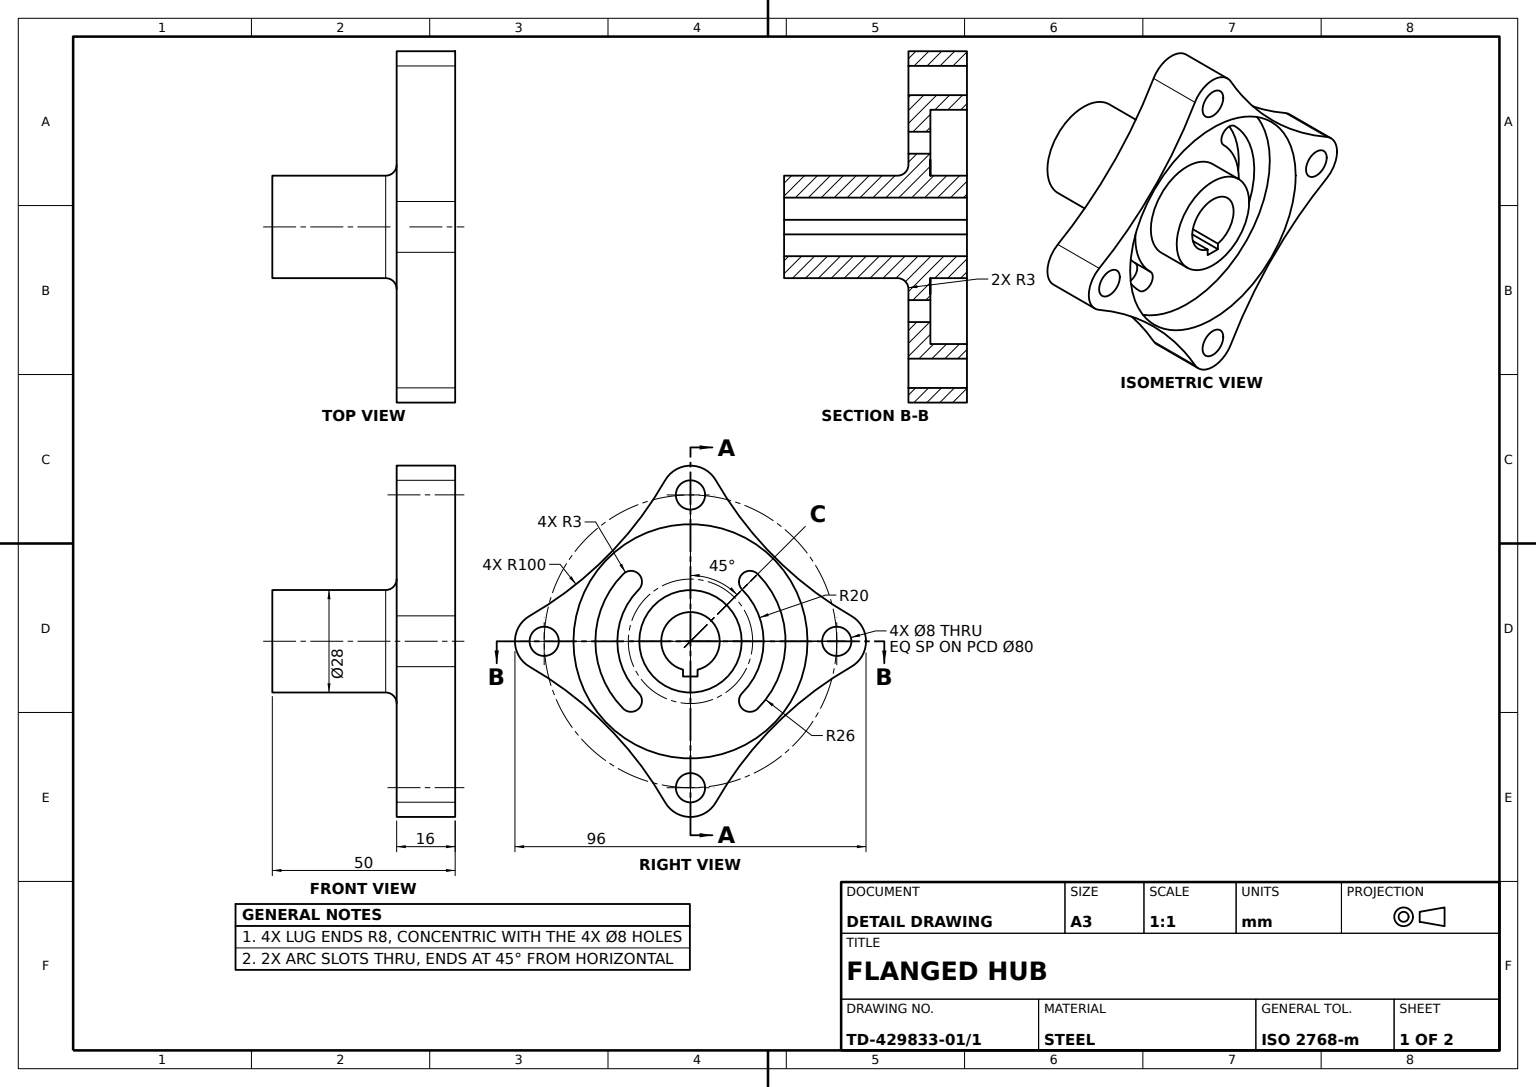
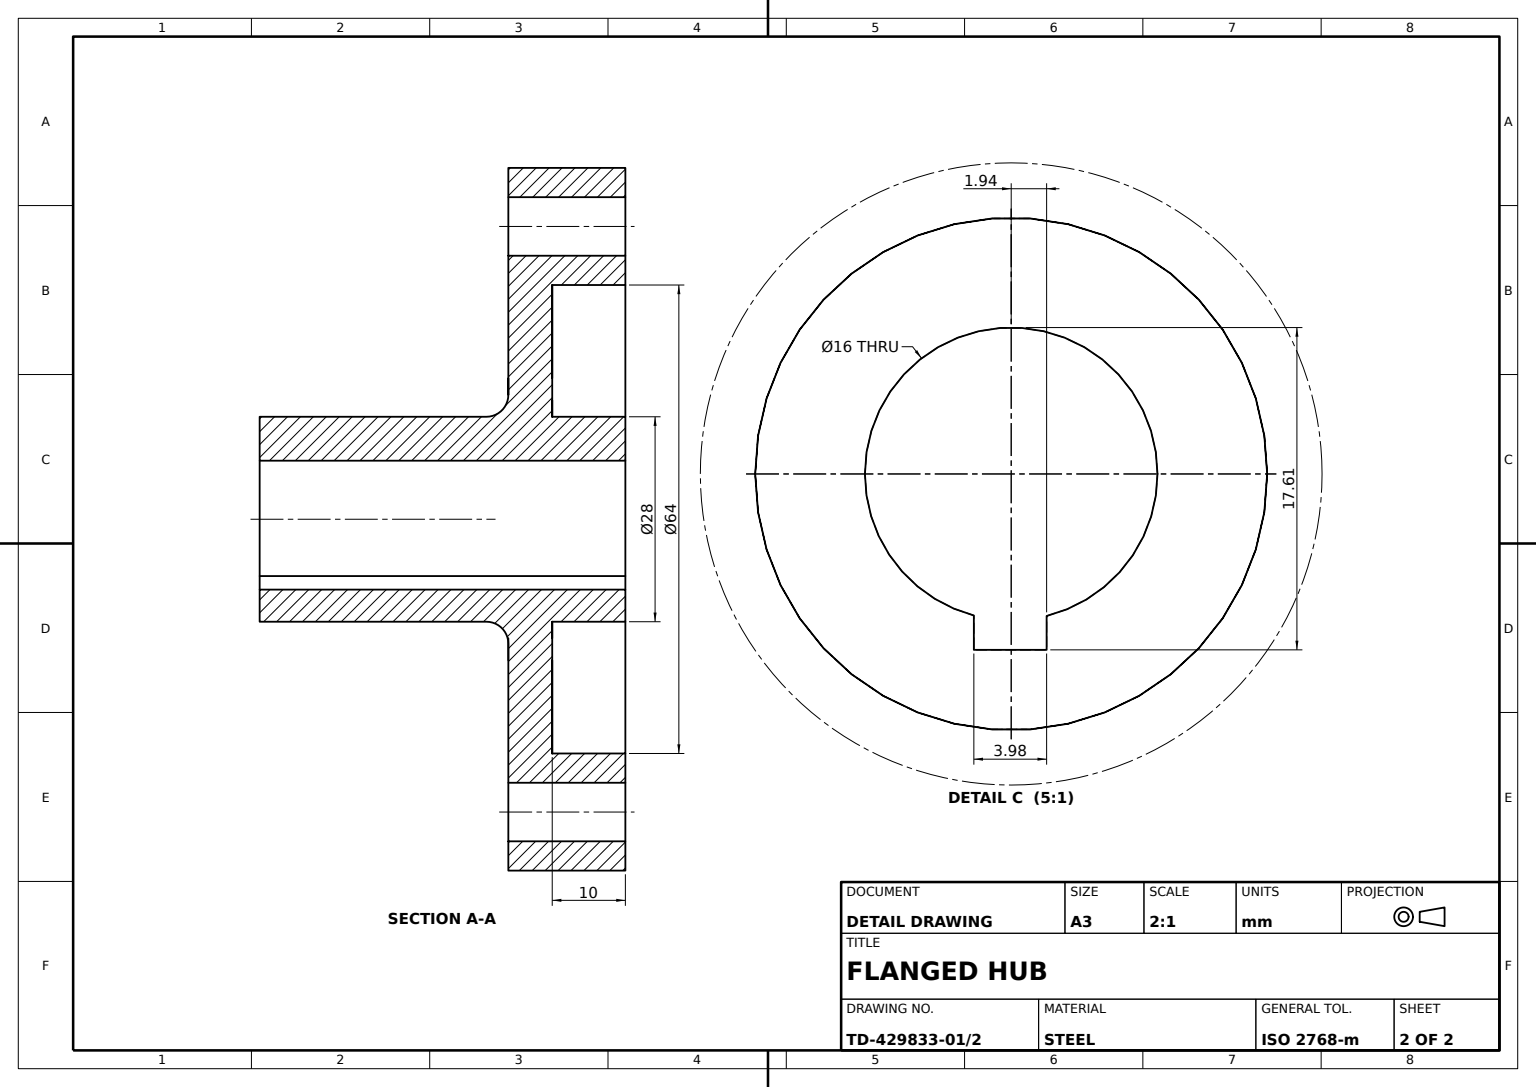
from build123d import *

# Parameters (mm, degrees)
FLANGE_PROFILE_SKETCH_R       = 4
SQUARE_FLANGE_100X16_DEPTH    = 16
RECESS_SKETCH_64_R            = 32
RECESS_64X10_DEPTH            = 10
HUB_BOSS_28_REACH             = 70.615
HUB_SKETCH_28_R               = 14
HUB_BOSS_28_DIRECTION_2_DEPTH = 40
HUB_FILLET_R3_R               = 3
KEYED_BORE_DEPTH              = 85.308955633
ARC_SLOTS_REACH               = 80.791


with BuildPart() as part:
    # Flange Profile Sketch → Square Flange 100x16 (new body)
    with BuildSketch(Plane(origin=(0, 0, 0), x_dir=(1, 0, 0), z_dir=(0, 1, 0))):
        with BuildLine():
            ThreePointArc((43.977933562, -6.940896525), (48, 0), (43.977933562, 6.940896525))
            ThreePointArc((43.977933562, 6.940896525), (22.991424972, 22.991424972), (6.940896525, 43.977933562))
            ThreePointArc((6.940896525, 43.977933562), (0, 48), (-6.940896525, 43.977933562))
            ThreePointArc((-6.940896525, 43.977933562), (-22.991424972, 22.991424972), (-43.977933562, 6.940896525))
            ThreePointArc((-43.977933562, 6.940896525), (-48, 0), (-43.977933562, -6.940896525))
            ThreePointArc((-43.977933562, -6.940896525), (-22.991424972, -22.991424972), (-6.940896525, -43.977933562))
            ThreePointArc((-6.940896525, -43.977933562), (0, -48), (6.940896525, -43.977933562))
            ThreePointArc((6.940896525, -43.977933562), (22.991424972, -22.991424972), (43.977933562, -6.940896525))
        make_face()
        with Locations(Location((40, 0, 0), (0, 0, 270))):
            Circle(FLANGE_PROFILE_SKETCH_R, mode=Mode.SUBTRACT)
        with Locations(Location((0, -40, 0), (0, 0, 270))):
            Circle(FLANGE_PROFILE_SKETCH_R, mode=Mode.SUBTRACT)
        with Locations(Location((-40, 0, 0), (0, 0, 270))):
            Circle(FLANGE_PROFILE_SKETCH_R, mode=Mode.SUBTRACT)
        with Locations(Location((0, 40, 0), (0, 0, 270))):
            Circle(FLANGE_PROFILE_SKETCH_R, mode=Mode.SUBTRACT)
    extrude(amount=SQUARE_FLANGE_100X16_DEPTH)

    # Recess Sketch Ø64 → Recess Ø64x10 (cut)
    with BuildSketch(Plane(origin=(0, 16, 0), x_dir=(1, 0, 0), z_dir=(0, 1, 0))):
        with Locations(Location((0, 0, 0), (0, 0, 270))):
            Circle(RECESS_SKETCH_64_R)
    extrude(amount=-RECESS_64X10_DEPTH, mode=Mode.SUBTRACT)

    # Hub Boss Ø28: up to this face of the body (flat: up to its plane)
    hub_boss_28_end = Plane(part.part.faces().sort_by_distance((22.895424972, 16, 22.895424972))[0])
    # Hub Sketch Ø28 → Hub Boss Ø28 (add, up to the picked face)
    with BuildSketch(Plane(origin=(0, 6, 0), x_dir=(1, 0, 0), z_dir=(0, 1, 0)), mode=Mode.PRIVATE) as hub_boss_28_sk1:
        with Locations(Location((0, 0, 0), (0, 0, 270))):
            Circle(HUB_SKETCH_28_R)
    hub_boss_28_tool1 = split(extrude(hub_boss_28_sk1.sketch, amount=HUB_BOSS_28_REACH, mode=Mode.PRIVATE), bisect_by=hub_boss_28_end, keep=Keep.BOTH, mode=Mode.PRIVATE)
    add(hub_boss_28_tool1.solids().sort_by(Axis((0, 6, 0), (0, 1, 0)))[0])

    # Hub Sketch Ø28 → Hub Boss Ø28 direction 2 (add)
    with BuildSketch(Plane(origin=(0, 6, 0), x_dir=(1, 0, 0), z_dir=(0, 1, 0))):
        with Locations(Location((0, 0, 0), (0, 0, 270))):
            Circle(HUB_SKETCH_28_R)
    extrude(amount=-HUB_BOSS_28_DIRECTION_2_DEPTH)

    # Hub Fillet R3
    hub_fillet_r3_edges = [part.edges().sort_by_distance(p)[0] for p in [
        (0, 0, -14),
    ]]
    fillet(hub_fillet_r3_edges, radius=HUB_FILLET_R3_R)

    # Keyed Bore Sketch → Keyed Bore (cut, through all)
    with BuildSketch(Plane(origin=(0, 16, 0), x_dir=(1, 0, 0), z_dir=(0, 1, 0))):
        with BuildLine():
            Line((9.611830035, 0), (9.611830035, 1.937522775))
            Line((9.611830035, 1.937522775), (7.761830035, 1.937522775))
            ThreePointArc((7.761830035, 1.937522775), (-7.999816529, 0.054180315), (7.73487471, -2.042477225))
            Line((7.73487471, -2.042477225), (9.611830035, -2.042477225))
            Line((9.611830035, -2.042477225), (9.611830035, 0))
        make_face()
    extrude(amount=-KEYED_BORE_DEPTH, mode=Mode.SUBTRACT)

    # Arc Slots Sketch → Arc Slots (cut, up to next)
    with BuildSketch(Plane(origin=(0, 6, 0), x_dir=(1, 0, 0), z_dir=(0, 1, 0)), mode=Mode.PRIVATE) as arc_slots_sk1:
        with BuildLine():
            ThreePointArc((18.384776311, 18.384776311), (0, 26), (-18.384776311, 18.384776311))
            ThreePointArc((-18.384776311, 18.384776311), (-18.384776311, 14.142135624), (-14.142135624, 14.142135624))
            ThreePointArc((-14.142135624, 14.142135624), (0, 20), (14.142135624, 14.142135624))
            ThreePointArc((14.142135624, 14.142135624), (18.384776311, 14.142135624), (18.384776311, 18.384776311))
        make_face()
    arc_slots_tool1 = extrude(arc_slots_sk1.sketch, amount=-ARC_SLOTS_REACH, mode=Mode.PRIVATE) & part.part
    # Arc Slots Sketch → Arc Slots (cut, up to next)
    with BuildSketch(Plane(origin=(0, 6, 0), x_dir=(1, 0, 0), z_dir=(0, 1, 0)), mode=Mode.PRIVATE) as arc_slots_sk2:
        with BuildLine():
            ThreePointArc((18.384776311, -18.384776311), (0, -26), (-18.384776311, -18.384776311))
            ThreePointArc((-18.384776311, -18.384776311), (-18.384776311, -14.142135624), (-14.142135624, -14.142135624))
            ThreePointArc((-14.142135624, -14.142135624), (0, -20), (14.142135624, -14.142135624))
            ThreePointArc((14.142135624, -14.142135624), (18.384776311, -14.142135624), (18.384776311, -18.384776311))
        make_face()
    arc_slots_tool2 = extrude(arc_slots_sk2.sketch, amount=-ARC_SLOTS_REACH, mode=Mode.PRIVATE) & part.part
    add(arc_slots_tool1.solids().sort_by_distance((0, 6, -20.194527))[0], mode=Mode.SUBTRACT)
    add(arc_slots_tool2.solids().sort_by_distance((0, 6, 20.194527))[0], mode=Mode.SUBTRACT)


solid = part.part
